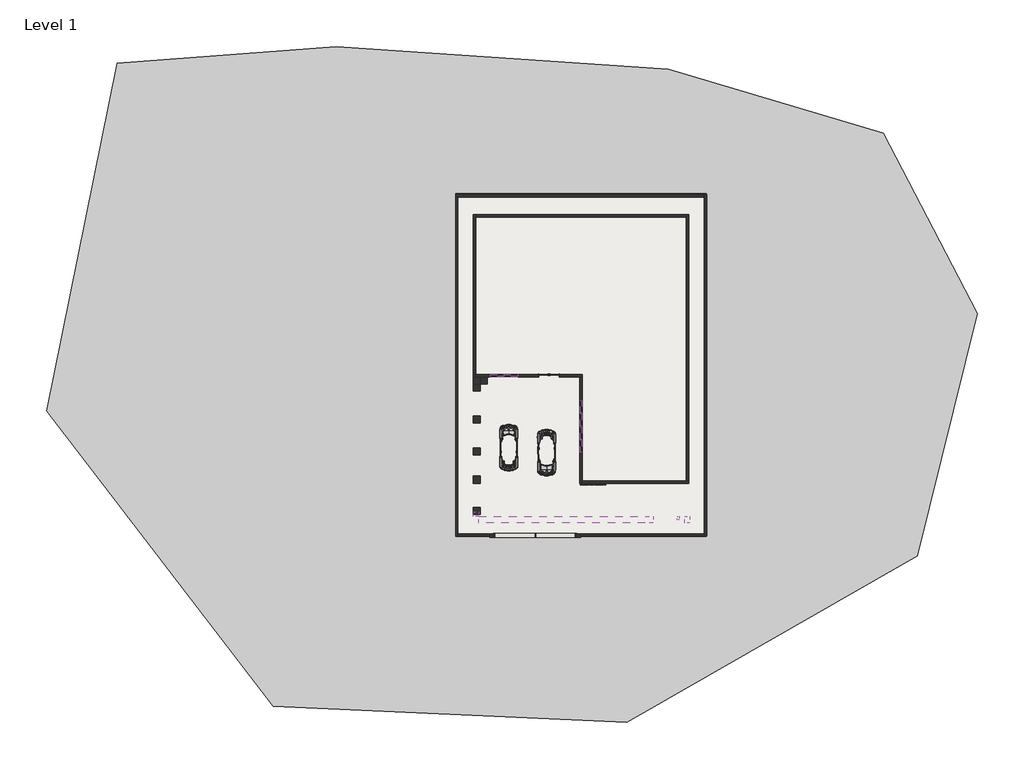
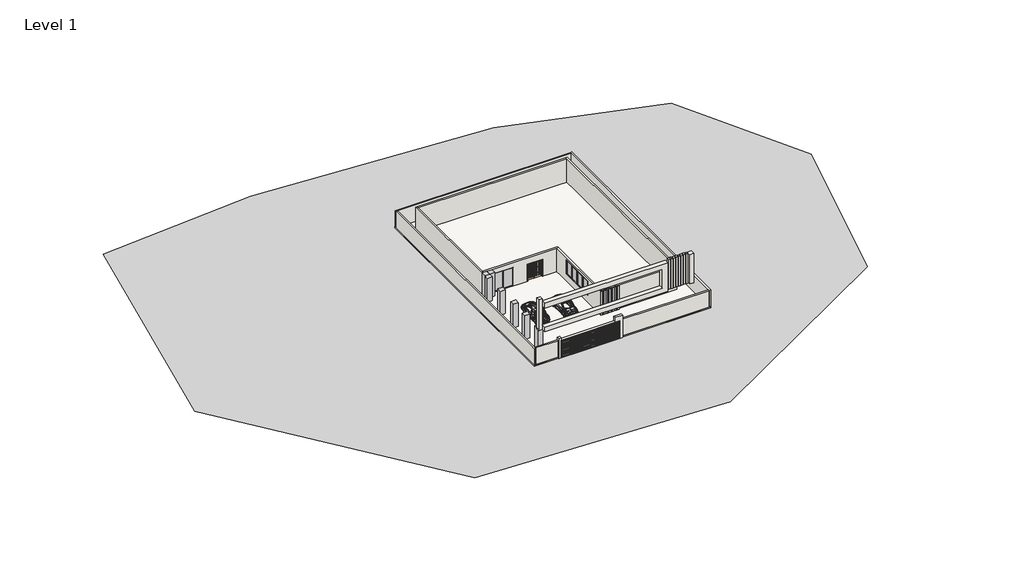
# One storey, incomplete: 20 members, 20 walls, 18 columns, 6 plates, 3 proxies, 1 door, 1 slab.
"""IFC4 building model written with IfcOpenShell, lengths in millimetres."""

from ifc_helpers import new_model, si_unit, frame, origin, origin_with_axes, place, context, project, spatial, polyline, outline, extrude, faceted_brep, triangles, transform, mapped, element, save
from components import rpc_beetle_rpc_beetle_3ce7ba48, m_rectangular_column_610_x_610mm_b887bf16, door_2f318157, rectangular_mullion_50_x_150mm_a98d9a75, rectangular_mullion_50_x_150mm_4a8db126, rectangular_mullion_50_x_150mm_7b2d4eb8, rectangular_mullion_50_x_150mm_561fbe3c, rectangular_mullion_50_x_150mm_8c42de37, rectangular_mullion_50_x_150mm_71d0ff5f, rectangular_mullion_50_x_150mm_c76b6149, system_panel_glazed_3787533d, system_panel_glazed_0469dc57, system_panel_glazed_71021e01, walls_1_walls_1_ac2cf788, walls_10_walls_9_f4ffd68b, walls_2_walls_2_f87d77c0, walls_4_walls_1_0671908a, walls_5_walls_5_96d48458, walls_6_walls_6_895ef20a, walls_7_walls_7_225e37e1, walls_8_walls_8_394d44dd, walls_9_walls_9_57911b2c

model = new_model("IFC4")

# Units and contexts
model_context = context("Model", 3, world=origin())
ifc_project = project(units=[si_unit("LENGTHUNIT", "METRE", prefix="MILLI")], contexts=[model_context])

# Site, building, storey
site = spatial("IfcSite", under=ifc_project)
building = spatial("IfcBuilding", under=site)
storey = spatial("IfcBuildingStorey", under=building, Name="Level 1", Elevation=0.0)

# Proxies
placement = place(None, origin())
element("IfcBuildingElementProxy", 1, Name="Building Element Proxy", at=placement, inside=storey, context=model_context, shape_type="Tessellation", body=[
    triangles([(-45355.9291992, -6804.9148682, -152.4), (-25904.1653503, -32148.7051208, -152.4), (4443.8121849, -33520.8213684, -152.4), (29384.0389893, -19234.671286, -152.4), (34549.651593, 1589.206921, -152.4), (26478.3814636, 17086.0466217, -152.4), (7995.171286, 22574.5104492, -152.4), (-20496.4140381, 24511.6154663, -152.4), (-39302.4754395, 23058.7878662, -152.4)], [[1, 2, 8], [8, 9, 1], [2, 3, 8], [3, 4, 7], [7, 5, 6], [5, 7, 4], [3, 7, 8]], closed=False),
])
rpc_beetle_rpc_beetle_shape = rpc_beetle_rpc_beetle_3ce7ba48(model_context)
element("IfcBuildingElementProxy", 2, Name="RPC Beetle : RPC Beetle", ObjectType="RPC Beetle : RPC Beetle", at=placement, inside=storey, context=model_context, shape_type="MappedRepresentation", body=[
    mapped(rpc_beetle_rpc_beetle_shape, transform((-5680.022521, -11169.2177849, 0.0), x_axis=(1.0, 0.0, 0.0), y_axis=(0.0, 1.0, 0.0), z_axis=(0.0, 0.0, 1.0))),
])
element("IfcBuildingElementProxy", 3, Name="RPC Beetle : RPC Beetle", ObjectType="RPC Beetle : RPC Beetle", at=placement, inside=storey, context=model_context, shape_type="MappedRepresentation", body=[
    mapped(rpc_beetle_rpc_beetle_shape, transform((-2432.022521, -9140.4177849, 0.0), x_axis=(-1.0000000000000004, 0.0, 0.0), y_axis=(0.0, -1.0000000000000004, 0.0), z_axis=(0.0, 0.0, 1.0))),
])

# Columns
element("IfcColumn", 4, ObjectType="M_Rectangular Column : 610 x 610mm", at=placement, inside=storey, context=model_context, shape_type="SweptSolid", body=[
    extrude(outline(polyline([(-8118.222521, -4463.8177849), (-8728.222521, -4463.8177849), (-8728.222521, -3853.8177849), (-8728.022521, -3853.8177849), (-8728.022521, -3854.0177849), (-8528.022521, -3854.0177849), (-8118.222521, -3854.0177849), (-8118.222521, -4463.8177849)])), origin_with_axes(), (0.0, 0.0, 1.0), 3048.0),
])
element("IfcColumn", 5, ObjectType="M_Rectangular Column : 610 x 610mm", at=placement, inside=storey, context=model_context, shape_type="SweptSolid", body=[
    extrude(outline(polyline([(-7508.622521, -4463.8177849), (-8118.622521, -4463.8177849), (-8118.622521, -3854.0177849), (-7508.622521, -3854.0177849), (-7508.622521, -4463.8177849)])), origin_with_axes(), (0.0, 0.0, 1.0), 3048.0),
])
m_rectangular_column_610_x_610mm_shape = m_rectangular_column_610_x_610mm_b887bf16(model_context)
element("IfcColumn", 6, ObjectType="M_Rectangular Column : 610 x 610mm", at=placement, inside=storey, context=model_context, shape_type="MappedRepresentation", body=[
    mapped(m_rectangular_column_610_x_610mm_shape, transform((-8423.222521, -4768.4177849, 0.0), x_axis=(1.0, 0.0, 0.0), y_axis=(0.0, 1.0, 0.0), z_axis=(0.0, 0.0, 1.0))),
])
element("IfcColumn", 7, ObjectType="M_Rectangular Column : 610 x 610mm", at=placement, inside=storey, context=model_context, shape_type="MappedRepresentation", body=[
    mapped(m_rectangular_column_610_x_610mm_shape, transform((-8423.222521, -7511.6177849, 0.0), x_axis=(1.0, 0.0, 0.0), y_axis=(0.0, 1.0, 0.0), z_axis=(0.0, 0.0, 1.0))),
])
element("IfcColumn", 8, ObjectType="M_Rectangular Column : 610 x 610mm", at=placement, inside=storey, context=model_context, shape_type="MappedRepresentation", body=[
    mapped(m_rectangular_column_610_x_610mm_shape, transform((-8423.222521, -10254.8177849, 0.0), x_axis=(1.0, 0.0, 0.0), y_axis=(0.0, 1.0, 0.0), z_axis=(0.0, 0.0, 1.0))),
])
element("IfcColumn", 9, ObjectType="M_Rectangular Column : 610 x 610mm", at=placement, inside=storey, context=model_context, shape_type="MappedRepresentation", body=[
    mapped(m_rectangular_column_610_x_610mm_shape, transform((-8423.222521, -12693.2177849, 0.0), x_axis=(1.0, 0.0, 0.0), y_axis=(0.0, 1.0, 0.0), z_axis=(0.0, 0.0, 1.0))),
])
element("IfcColumn", 10, ObjectType="M_Rectangular Column : 610 x 610mm", at=placement, inside=storey, context=model_context, shape_type="MappedRepresentation", body=[
    mapped(m_rectangular_column_610_x_610mm_shape, transform((-8423.222521, -15385.6177849, 0.0), x_axis=(1.0, 0.0, 0.0), y_axis=(0.0, 1.0, 0.0), z_axis=(0.0, 0.0, 1.0))),
])
element("IfcColumn", 11, ObjectType="M_Rectangular Column : COL 2", at=placement, inside=storey, context=model_context, shape_type="SweptSolid", body=[
    extrude(outline(polyline([(592.177479, -12998.0177849), (592.177479, -13150.4177849), (439.777479, -13150.4177849), (439.777479, -12998.0177849), (592.177479, -12998.0177849)])), origin_with_axes(), (0.0, 0.0, 1.0), 3048.0),
])
element("IfcColumn", 12, ObjectType="M_Rectangular Column : COL 2", at=placement, inside=storey, context=model_context, shape_type="SweptSolid", body=[
    extrude(outline(polyline([(793.777479, -12998.0177849), (793.777479, -13150.4177849), (641.377479, -13150.4177849), (641.377479, -12998.0177849), (793.777479, -12998.0177849)])), origin_with_axes(), (0.0, 0.0, 1.0), 3048.0),
])
element("IfcColumn", 13, ObjectType="M_Rectangular Column : COL 2", at=placement, inside=storey, context=model_context, shape_type="SweptSolid", body=[
    extrude(outline(polyline([(996.977479, -12998.0177849), (996.977479, -13150.4177849), (844.577479, -13150.4177849), (844.577479, -12998.0177849), (996.977479, -12998.0177849)])), origin_with_axes(), (0.0, 0.0, 1.0), 3048.0),
])
element("IfcColumn", 14, ObjectType="M_Rectangular Column : COL 2", at=placement, inside=storey, context=model_context, shape_type="SweptSolid", body=[
    extrude(outline(polyline([(1200.177479, -12998.0177849), (1200.177479, -13150.4177849), (1047.777479, -13150.4177849), (1047.777479, -12998.0177849), (1200.177479, -12998.0177849)])), origin_with_axes(), (0.0, 0.0, 1.0), 3048.0),
])
element("IfcColumn", 15, ObjectType="M_Rectangular Column : COL 2", at=placement, inside=storey, context=model_context, shape_type="SweptSolid", body=[
    extrude(outline(polyline([(1403.377479, -12998.0177849), (1403.377479, -13150.4177849), (1250.977479, -13150.4177849), (1250.977479, -12998.0177849), (1403.377479, -12998.0177849)])), origin_with_axes(), (0.0, 0.0, 1.0), 3048.0),
])
element("IfcColumn", 16, ObjectType="M_Rectangular Column : COL 2", at=placement, inside=storey, context=model_context, shape_type="SweptSolid", body=[
    extrude(outline(polyline([(1606.577479, -12998.0177849), (1606.577479, -13150.4177849), (1454.177479, -13150.4177849), (1454.177479, -12998.0177849), (1606.577479, -12998.0177849)])), origin_with_axes(), (0.0, 0.0, 1.0), 3048.0),
])
element("IfcColumn", 17, ObjectType="M_Rectangular Column : COL 2", at=placement, inside=storey, context=model_context, shape_type="SweptSolid", body=[
    extrude(outline(polyline([(1835.177479, -12998.0177849), (1835.177479, -13150.4177849), (1682.777479, -13150.4177849), (1682.777479, -12998.0177849), (1835.177479, -12998.0177849)])), origin_with_axes(), (0.0, 0.0, 1.0), 3048.0),
])
element("IfcColumn", 18, ObjectType="M_Rectangular Column : COL 2", at=placement, inside=storey, context=model_context, shape_type="SweptSolid", body=[
    extrude(outline(polyline([(2038.377479, -12998.0177849), (2038.377479, -13150.4177849), (1885.977479, -13150.4177849), (1885.977479, -12998.0177849), (2038.377479, -12998.0177849)])), origin_with_axes(), (0.0, 0.0, 1.0), 3048.0),
])
element("IfcColumn", 19, ObjectType="M_Rectangular Column : COL 2", at=placement, inside=storey, context=model_context, shape_type="SweptSolid", body=[
    extrude(outline(polyline([(2241.577479, -12998.0177849), (2241.577479, -13150.4177849), (2089.177479, -13150.4177849), (2089.177479, -12998.0177849), (2241.577479, -12998.0177849)])), origin_with_axes(), (0.0, 0.0, 1.0), 3048.0),
])
element("IfcColumn", 20, ObjectType="M_Rectangular Column : COL 2", at=placement, inside=storey, context=model_context, shape_type="SweptSolid", body=[
    extrude(outline(polyline([(2444.777479, -12998.0177849), (2444.777479, -13150.4177849), (2292.377479, -13150.4177849), (2292.377479, -12998.0177849), (2444.777479, -12998.0177849)])), origin_with_axes(), (0.0, 0.0, 1.0), 3048.0),
])
element("IfcColumn", 21, ObjectType="M_Rectangular Column : COL 2", at=placement, inside=storey, context=model_context, shape_type="SweptSolid", body=[
    extrude(outline(polyline([(2647.977479, -12998.0177849), (2647.977479, -13150.4177849), (2495.577479, -13150.4177849), (2495.577479, -12998.0177849), (2647.977479, -12998.0177849)])), origin_with_axes(), (0.0, 0.0, 1.0), 3048.0),
])

# Door
door_shape = door_2f318157(model_context)
element("IfcDoor", 22, ObjectType="Door-Interior-Double-Full Glass-Wood : 68\" x 84\"", at=placement, inside=storey, context=model_context, shape_type="MappedRepresentation", body=[
    mapped(door_shape, transform((-2227.222521, -3750.8427849, 0.0), x_axis=(1.0, 0.0, 0.0), y_axis=(0.0, 1.0, 0.0), z_axis=(0.0, 0.0, 1.0))),
])

# Members
rectangular_mullion_50_x_150mm_shape = rectangular_mullion_50_x_150mm_a98d9a75(model_context)
element("IfcMember", 23, ObjectType="Rectangular Mullion : 50 x 150mm", at=placement, inside=storey, context=model_context, shape_type="MappedRepresentation", body=[
    mapped(rectangular_mullion_50_x_150mm_shape, transform((-6089.622521, -3754.0177849, 0.0), x_axis=(1.0, 0.0, 0.0), y_axis=(0.0, -1.0, 0.0), z_axis=(0.0, 0.0, -1.0))),
])
rectangular_mullion_50_x_150mm_2_shape = rectangular_mullion_50_x_150mm_4a8db126(model_context)
element("IfcMember", 24, ObjectType="Rectangular Mullion : 50 x 150mm", at=placement, inside=storey, context=model_context, shape_type="MappedRepresentation", body=[
    mapped(rectangular_mullion_50_x_150mm_2_shape, transform((-7308.822521, -3754.0177849, 2438.4), x_axis=(-1.0, 0.0, 0.0), y_axis=(0.0, -1.0, 0.0), z_axis=(0.0, 0.0, 1.0))),
])
element("IfcMember", 25, ObjectType="Rectangular Mullion : 50 x 150mm", at=placement, inside=storey, context=model_context, shape_type="MappedRepresentation", body=[
    mapped(rectangular_mullion_50_x_150mm_2_shape, transform((-4870.422521, -3754.0177849, 0.0), x_axis=(1.0, 0.0, 0.0), y_axis=(0.0, -1.0, 0.0), z_axis=(0.0, 0.0, -1.0))),
])
rectangular_mullion_50_x_150mm_3_shape = rectangular_mullion_50_x_150mm_7b2d4eb8(model_context)
element("IfcMember", 26, ObjectType="Rectangular Mullion : 50 x 150mm", at=placement, inside=storey, context=model_context, shape_type="MappedRepresentation", body=[
    mapped(rectangular_mullion_50_x_150mm_3_shape, transform((-4920.422521, -3754.0177849, 2438.4), x_axis=(0.0, 0.0, 1.0), y_axis=(0.0, -1.0, 0.0), z_axis=(1.0, 0.0, 0.0))),
])
element("IfcMember", 27, ObjectType="Rectangular Mullion : 50 x 150mm", at=placement, inside=storey, context=model_context, shape_type="MappedRepresentation", body=[
    mapped(rectangular_mullion_50_x_150mm_3_shape, transform((-6114.622521, -3754.0177849, 2438.4), x_axis=(0.0, 0.0, 1.0), y_axis=(0.0, -1.0, 0.0), z_axis=(1.0, 0.0, 0.0))),
])
element("IfcMember", 28, ObjectType="Rectangular Mullion : 50 x 150mm", at=placement, inside=storey, context=model_context, shape_type="MappedRepresentation", body=[
    mapped(rectangular_mullion_50_x_150mm_3_shape, transform((-7258.822521, -3754.0177849, 0.0), x_axis=(0.0, 0.0, -1.0), y_axis=(0.0, -1.0, 0.0), z_axis=(-1.0, 0.0, 0.0))),
])
element("IfcMember", 29, ObjectType="Rectangular Mullion : 50 x 150mm", at=placement, inside=storey, context=model_context, shape_type="MappedRepresentation", body=[
    mapped(rectangular_mullion_50_x_150mm_3_shape, transform((-6064.622521, -3754.0177849, 0.0), x_axis=(0.0, 0.0, -1.0), y_axis=(0.0, -1.0, 0.0), z_axis=(-1.0, 0.0, 0.0))),
])
rectangular_mullion_50_x_150mm_4_shape = rectangular_mullion_50_x_150mm_561fbe3c(model_context)
element("IfcMember", 30, ObjectType="Rectangular Mullion : 50 x 150mm", at=placement, inside=storey, context=model_context, shape_type="MappedRepresentation", body=[
    mapped(rectangular_mullion_50_x_150mm_4_shape, transform((515.977479, -10357.2177849, 2743.2), x_axis=(0.0, 0.0, 1.0), y_axis=(-1.0, 0.0, 0.0), z_axis=(0.0, -1.0, 0.0))),
])
element("IfcMember", 31, ObjectType="Rectangular Mullion : 50 x 150mm", at=placement, inside=storey, context=model_context, shape_type="MappedRepresentation", body=[
    mapped(rectangular_mullion_50_x_150mm_4_shape, transform((515.977479, -6953.2177849, 2743.2), x_axis=(0.0, 0.0, 1.0), y_axis=(-1.0, 0.0, 0.0), z_axis=(0.0, -1.0, 0.0))),
])
element("IfcMember", 32, ObjectType="Rectangular Mullion : 50 x 150mm", at=placement, inside=storey, context=model_context, shape_type="MappedRepresentation", body=[
    mapped(rectangular_mullion_50_x_150mm_4_shape, transform((515.977479, -5885.2177849, 914.4), x_axis=(0.0, 0.0, -1.0), y_axis=(-1.0, 0.0, 0.0), z_axis=(0.0, 1.0, 0.0))),
])
element("IfcMember", 33, ObjectType="Rectangular Mullion : 50 x 150mm", at=placement, inside=storey, context=model_context, shape_type="MappedRepresentation", body=[
    mapped(rectangular_mullion_50_x_150mm_4_shape, transform((515.977479, -9289.2177849, 914.4), x_axis=(0.0, 0.0, -1.0), y_axis=(-1.0, 0.0, 0.0), z_axis=(0.0, 1.0, 0.0))),
])
rectangular_mullion_50_x_150mm_5_shape = rectangular_mullion_50_x_150mm_8c42de37(model_context)
element("IfcMember", 34, ObjectType="Rectangular Mullion : 50 x 150mm", at=placement, inside=storey, context=model_context, shape_type="MappedRepresentation", body=[
    mapped(rectangular_mullion_50_x_150mm_5_shape, transform((515.977479, -8121.2177849, 914.4), x_axis=(0.0, -1.0, 0.0), y_axis=(-1.0, 0.0, 0.0), z_axis=(0.0, 0.0, -1.0))),
])
element("IfcMember", 35, ObjectType="Rectangular Mullion : 50 x 150mm", at=placement, inside=storey, context=model_context, shape_type="MappedRepresentation", body=[
    mapped(rectangular_mullion_50_x_150mm_5_shape, transform((515.977479, -6978.2177849, 914.4), x_axis=(0.0, -1.0, 0.0), y_axis=(-1.0, 0.0, 0.0), z_axis=(0.0, 0.0, -1.0))),
])
element("IfcMember", 36, ObjectType="Rectangular Mullion : 50 x 150mm", at=placement, inside=storey, context=model_context, shape_type="MappedRepresentation", body=[
    mapped(rectangular_mullion_50_x_150mm_5_shape, transform((515.977479, -9264.2177849, 914.4), x_axis=(0.0, -1.0, 0.0), y_axis=(-1.0, 0.0, 0.0), z_axis=(0.0, 0.0, -1.0))),
])
rectangular_mullion_50_x_150mm_6_shape = rectangular_mullion_50_x_150mm_71d0ff5f(model_context)
element("IfcMember", 37, ObjectType="Rectangular Mullion : 50 x 150mm", at=placement, inside=storey, context=model_context, shape_type="MappedRepresentation", body=[
    mapped(rectangular_mullion_50_x_150mm_6_shape, transform((515.977479, -8146.2177849, 914.4), x_axis=(0.0, 0.0, -1.0), y_axis=(-1.0, 0.0, 0.0), z_axis=(0.0, 1.0, 0.0))),
])
element("IfcMember", 38, ObjectType="Rectangular Mullion : 50 x 150mm", at=placement, inside=storey, context=model_context, shape_type="MappedRepresentation", body=[
    mapped(rectangular_mullion_50_x_150mm_6_shape, transform((515.977479, -7003.2177849, 914.4), x_axis=(0.0, 0.0, -1.0), y_axis=(-1.0, 0.0, 0.0), z_axis=(0.0, 1.0, 0.0))),
])
element("IfcMember", 39, ObjectType="Rectangular Mullion : 50 x 150mm", at=placement, inside=storey, context=model_context, shape_type="MappedRepresentation", body=[
    mapped(rectangular_mullion_50_x_150mm_6_shape, transform((515.977479, -8096.2177849, 2743.2), x_axis=(0.0, 0.0, 1.0), y_axis=(-1.0, 0.0, 0.0), z_axis=(0.0, -1.0, 0.0))),
])
element("IfcMember", 40, ObjectType="Rectangular Mullion : 50 x 150mm", at=placement, inside=storey, context=model_context, shape_type="MappedRepresentation", body=[
    mapped(rectangular_mullion_50_x_150mm_6_shape, transform((515.977479, -9239.2177849, 2743.2), x_axis=(0.0, 0.0, 1.0), y_axis=(-1.0, 0.0, 0.0), z_axis=(0.0, -1.0, 0.0))),
])
rectangular_mullion_50_x_150mm_7_shape = rectangular_mullion_50_x_150mm_c76b6149(model_context)
element("IfcMember", 41, ObjectType="Rectangular Mullion : 50 x 150mm", at=placement, inside=storey, context=model_context, shape_type="MappedRepresentation", body=[
    mapped(rectangular_mullion_50_x_150mm_7_shape, transform((515.977479, -5835.2177849, 2743.2), x_axis=(0.0, 1.0, 0.0), y_axis=(-1.0, 0.0, 0.0), z_axis=(0.0, 0.0, 1.0))),
])
element("IfcMember", 42, ObjectType="Rectangular Mullion : 50 x 150mm", at=placement, inside=storey, context=model_context, shape_type="MappedRepresentation", body=[
    mapped(rectangular_mullion_50_x_150mm_7_shape, transform((515.977479, -10407.2177849, 914.4), x_axis=(0.0, -1.0, 0.0), y_axis=(-1.0, 0.0, 0.0), z_axis=(0.0, 0.0, -1.0))),
])

# Plates
system_panel_glazed_shape = system_panel_glazed_3787533d(model_context)
element("IfcPlate", 43, ObjectType="System Panel : Glazed", at=placement, inside=storey, context=model_context, shape_type="MappedRepresentation", body=[
    mapped(system_panel_glazed_shape, transform((-6686.722521, -3754.0177849, 50.0), x_axis=(1.0, 0.0, 0.0), y_axis=(0.0, 1.0, 0.0), z_axis=(0.0, 0.0, 1.0))),
])
element("IfcPlate", 44, ObjectType="System Panel : Glazed", at=placement, inside=storey, context=model_context, shape_type="MappedRepresentation", body=[
    mapped(system_panel_glazed_shape, transform((-5492.522521, -3754.0177849, 50.0), x_axis=(1.0, 0.0, 0.0), y_axis=(0.0, 1.0, 0.0), z_axis=(0.0, 0.0, 1.0))),
])
system_panel_glazed_2_shape = system_panel_glazed_0469dc57(model_context)
element("IfcPlate", 45, ObjectType="System Panel : Glazed", at=placement, inside=storey, context=model_context, shape_type="MappedRepresentation", body=[
    mapped(system_panel_glazed_2_shape, transform((515.977479, -6419.2177849, 964.4), x_axis=(0.0, -1.0, 0.0), y_axis=(1.0, 0.0, 0.0), z_axis=(0.0, 0.0, 1.0))),
])
element("IfcPlate", 46, ObjectType="System Panel : Glazed", at=placement, inside=storey, context=model_context, shape_type="MappedRepresentation", body=[
    mapped(system_panel_glazed_2_shape, transform((515.977479, -9823.2177849, 964.4), x_axis=(0.0, -1.0, 0.0), y_axis=(1.0, 0.0, 0.0), z_axis=(0.0, 0.0, 1.0))),
])
system_panel_glazed_3_shape = system_panel_glazed_71021e01(model_context)
element("IfcPlate", 47, ObjectType="System Panel : Glazed", at=placement, inside=storey, context=model_context, shape_type="MappedRepresentation", body=[
    mapped(system_panel_glazed_3_shape, transform((515.977479, -8692.7177849, 964.4), x_axis=(0.0, -1.0, 0.0), y_axis=(1.0, 0.0, 0.0), z_axis=(0.0, 0.0, 1.0))),
])
element("IfcPlate", 48, ObjectType="System Panel : Glazed", at=placement, inside=storey, context=model_context, shape_type="MappedRepresentation", body=[
    mapped(system_panel_glazed_3_shape, transform((515.977479, -7549.7177849, 964.4), x_axis=(0.0, -1.0, 0.0), y_axis=(1.0, 0.0, 0.0), z_axis=(0.0, 0.0, 1.0))),
])

# Slab
element("IfcSlab", 49, ObjectType="Generic 150mm", at=placement, inside=storey, context=model_context, shape_type="SweptSolid", body=[
    extrude(outline(polyline([(-10252.022521, 11890.7822151), (11283.977479, 11890.7822151), (11283.977479, -17570.0177849), (-10252.022521, -17570.0177849), (-10252.022521, 11890.7822151)])), frame((0.0, 0.0, -152.4), z_axis=(0.0, 0.0, 1.0), x_axis=(1.0, 0.0, 0.0)), (0.0, 0.0, 1.0), 152.4),
])

# Walls
element("IfcWall", 50, ObjectType="Generic - 200mm", at=placement, inside=storey, context=model_context, shape_type="Brep", body=[
    faceted_brep([(-8728.022521, 10061.9822151, 0.0), (-8728.022521, -3853.8177849, 0.0), (-8728.022521, -3854.0177849, 0.0), (-8728.022521, -3854.0177849, 3048.0), (-8728.022521, -3853.8177849, 3048.0), (-8728.022521, 10061.9822151, 3048.0), (-8528.022521, 10061.9822151, 0.0), (-8528.022521, 10061.9822151, 3048.0), (-8528.022521, 9861.9822151, 3048.0), (-8528.022521, -3654.0177849, 3048.0), (-8528.022521, -3854.0177849, 3048.0), (-8528.022521, -3854.0177849, 0.0), (-8528.022521, -3654.0177849, 0.0), (-8528.022521, 9861.9822151, 0.0)], [[[0, 1, 2, 3, 4, 5]], [[6, 7, 8, 9, 10, 11, 12, 13]], [[2, 1, 0, 6, 13, 12, 11]], [[5, 4, 3, 10, 9, 8, 7]], [[3, 2, 11, 10]], [[0, 5, 7, 6]]]),
])
element("IfcWall", 51, ObjectType="Generic - 200mm", at=placement, inside=storey, context=model_context, shape_type="Brep", body=[
    faceted_brep([(615.977479, -3854.0177849, 3048.0), (415.977479, -3854.0177849, 3048.0), (-7508.622521, -3854.0177849, 3048.0), (-8118.222521, -3854.0177849, 3048.0), (-8118.622521, -3854.0177849, 3048.0), (-8528.022521, -3854.0177849, 3048.0), (-8528.022521, -3854.0177849, 0.0), (-8118.622521, -3854.0177849, 0.0), (-8118.222521, -3854.0177849, 0.0), (-7508.622521, -3854.0177849, 0.0), (-7308.822521, -3854.0177849, 0.0), (-7308.822521, -3854.0177849, 2438.4), (-4870.422521, -3854.0177849, 2438.4), (-4870.422521, -3854.0177849, 0.0), (-3116.222521, -3854.0177849, 0.0), (-3116.222521, -3854.0177849, 2159.0), (-1338.222521, -3854.0177849, 2159.0), (-1338.222521, -3854.0177849, 0.0), (415.977479, -3854.0177849, 0.0), (615.977479, -3854.0177849, 0.0), (-8528.022521, -3654.0177849, 3048.0), (615.977479, -3654.0177849, 3048.0), (615.977479, -3654.0177849, 0.0), (-1338.222521, -3654.0177849, 0.0), (-1338.222521, -3654.0177849, 2159.0), (-3116.222521, -3654.0177849, 2159.0), (-3116.222521, -3654.0177849, 0.0), (-4870.422521, -3654.0177849, 0.0), (-4870.422521, -3654.0177849, 2438.4), (-7308.822521, -3654.0177849, 2438.4), (-7308.822521, -3654.0177849, 0.0), (-8528.022521, -3654.0177849, 0.0)], [[[0, 1, 2, 3, 4, 5, 6, 7, 8, 9, 10, 11, 12, 13, 14, 15, 16, 17, 18, 19]], [[20, 21, 22, 23, 24, 25, 26, 27, 28, 29, 30, 31]], [[6, 31, 30, 10, 9, 8, 7]], [[22, 19, 18, 17, 23]], [[13, 27, 26, 14]], [[5, 4, 3, 2, 1, 0, 21, 20]], [[6, 5, 20, 31]], [[0, 19, 22, 21]], [[29, 11, 10, 30]], [[11, 29, 28, 12]], [[12, 28, 27, 13]], [[16, 24, 23, 17]], [[24, 16, 15, 25]], [[25, 15, 14, 26]]]),
])
element("IfcWall", 52, ObjectType="Generic - 200mm", at=placement, inside=storey, context=model_context, shape_type="Brep", body=[
    faceted_brep([(415.977479, -3854.0177849, 0.0), (415.977479, -12998.0177849, 0.0), (415.977479, -12998.0177849, 3048.0), (415.977479, -3854.0177849, 3048.0), (415.977479, -5835.2177849, 914.4), (415.977479, -5835.2177849, 2743.2), (415.977479, -10407.2177849, 2743.2), (415.977479, -10407.2177849, 914.4), (615.977479, -12998.0177849, 0.0), (615.977479, -12798.0177849, 0.0), (615.977479, -3854.0177849, 0.0), (615.977479, -3854.0177849, 3048.0), (615.977479, -12798.0177849, 3048.0), (615.977479, -12998.0177849, 3048.0), (615.977479, -5835.2177849, 2743.2), (615.977479, -5835.2177849, 914.4), (615.977479, -10407.2177849, 914.4), (615.977479, -10407.2177849, 2743.2), (592.177479, -12998.0177849, 0.0), (439.777479, -12998.0177849, 0.0), (439.777479, -12998.0177849, 3048.0), (592.177479, -12998.0177849, 3048.0)], [[[0, 1, 2, 3], [4, 5, 6, 7]], [[8, 9, 10, 11, 12, 13], [14, 15, 16, 17]], [[1, 0, 10, 9, 8, 18, 19]], [[3, 2, 20, 21, 13, 12, 11]], [[0, 3, 11, 10]], [[2, 1, 19, 18, 8, 13, 21, 20]], [[4, 15, 14, 5]], [[5, 14, 17, 6]], [[6, 17, 16, 7]], [[15, 4, 7, 16]]]),
])
element("IfcWall", 53, ObjectType="Generic - 200mm", at=placement, inside=storey, context=model_context, shape_type="Brep", body=[
    faceted_brep([(615.977479, -12998.0177849, 0.0), (641.377479, -12998.0177849, 0.0), (793.777479, -12998.0177849, 0.0), (844.577479, -12998.0177849, 0.0), (996.977479, -12998.0177849, 0.0), (1047.777479, -12998.0177849, 0.0), (1200.177479, -12998.0177849, 0.0), (1250.977479, -12998.0177849, 0.0), (1403.377479, -12998.0177849, 0.0), (1454.177479, -12998.0177849, 0.0), (1606.577479, -12998.0177849, 0.0), (1682.777479, -12998.0177849, 0.0), (1835.177479, -12998.0177849, 0.0), (1885.977479, -12998.0177849, 0.0), (2038.377479, -12998.0177849, 0.0), (2089.177479, -12998.0177849, 0.0), (2241.577479, -12998.0177849, 0.0), (2292.377479, -12998.0177849, 0.0), (2444.777479, -12998.0177849, 0.0), (2495.577479, -12998.0177849, 0.0), (2647.977479, -12998.0177849, 0.0), (9759.977479, -12998.0177849, 0.0), (9759.977479, -12998.0177849, 3048.0), (2647.977479, -12998.0177849, 3048.0), (2495.577479, -12998.0177849, 3048.0), (2444.777479, -12998.0177849, 3048.0), (2292.377479, -12998.0177849, 3048.0), (2241.577479, -12998.0177849, 3048.0), (2089.177479, -12998.0177849, 3048.0), (2038.377479, -12998.0177849, 3048.0), (1885.977479, -12998.0177849, 3048.0), (1835.177479, -12998.0177849, 3048.0), (1682.777479, -12998.0177849, 3048.0), (1606.577479, -12998.0177849, 3048.0), (1454.177479, -12998.0177849, 3048.0), (1403.377479, -12998.0177849, 3048.0), (1250.977479, -12998.0177849, 3048.0), (1200.177479, -12998.0177849, 3048.0), (1047.777479, -12998.0177849, 3048.0), (996.977479, -12998.0177849, 3048.0), (844.577479, -12998.0177849, 3048.0), (793.777479, -12998.0177849, 3048.0), (641.377479, -12998.0177849, 3048.0), (615.977479, -12998.0177849, 3048.0), (615.977479, -12798.0177849, 0.0), (615.977479, -12798.0177849, 3048.0), (9559.977479, -12798.0177849, 3048.0), (9759.977479, -12798.0177849, 3048.0), (9759.977479, -12798.0177849, 0.0), (9559.977479, -12798.0177849, 0.0)], [[[0, 1, 2, 3, 4, 5, 6, 7, 8, 9, 10, 11, 12, 13, 14, 15, 16, 17, 18, 19, 20, 21, 22, 23, 24, 25, 26, 27, 28, 29, 30, 31, 32, 33, 34, 35, 36, 37, 38, 39, 40, 41, 42, 43]], [[44, 45, 46, 47, 48, 49]], [[21, 20, 19, 18, 17, 16, 15, 14, 13, 12, 11, 10, 9, 8, 7, 6, 5, 4, 3, 2, 1, 0, 44, 49, 48]], [[43, 42, 41, 40, 39, 38, 37, 36, 35, 34, 33, 32, 31, 30, 29, 28, 27, 26, 25, 24, 23, 22, 47, 46, 45]], [[0, 43, 45, 44]], [[22, 21, 48, 47]]]),
])
element("IfcWall", 54, ObjectType="Generic - 200mm", at=placement, inside=storey, context=model_context, shape_type="Brep", body=[
    faceted_brep([(9759.977479, -12798.0177849, 0.0), (9759.977479, 10061.9822151, 0.0), (9759.977479, 10061.9822151, 3048.0), (9759.977479, -12798.0177849, 3048.0), (9559.977479, -12798.0177849, 0.0), (9559.977479, -12798.0177849, 3048.0), (9559.977479, 9861.9822151, 3048.0), (9559.977479, 10061.9822151, 3048.0), (9559.977479, 10061.9822151, 0.0), (9559.977479, 9861.9822151, 0.0)], [[[0, 1, 2, 3]], [[4, 5, 6, 7, 8, 9]], [[1, 0, 4, 9, 8]], [[3, 2, 7, 6, 5]], [[0, 3, 5, 4]], [[2, 1, 8, 7]]]),
])
element("IfcWall", 55, ObjectType="Generic - 200mm", at=placement, inside=storey, context=model_context, shape_type="SweptSolid", body=[
    extrude(outline(polyline([(-8528.022521, 10061.9822151), (9559.977479, 10061.9822151), (9559.977479, 9861.9822151), (-8528.022521, 9861.9822151), (-8528.022521, 10061.9822151)])), origin_with_axes(), (0.0, 0.0, 1.0), 3048.0),
])
element("IfcWall", 56, ObjectType="Generic - 200mm", at=placement, inside=storey, context=model_context, shape_type="Brep", body=[
    faceted_brep([(11292.9366262, -17534.2834973, 0.0), (11292.9366262, 11774.1165027, 0.0), (11292.9366262, 11774.1165027, 2133.6), (11292.9366262, -17534.2834973, 2133.6), (11092.9366262, -17534.2834973, 0.0), (11092.9366262, -17534.2834973, 2133.6), (11092.9366262, -17334.2834973, 2133.6), (11092.9366262, 11574.1165027, 2133.6), (11092.9366262, 11774.1165027, 2133.6), (11092.9366262, 11774.1165027, 0.0), (11092.9366262, 11574.1165027, 0.0), (11092.9366262, -17334.2834973, 0.0)], [[[0, 1, 2, 3]], [[4, 5, 6, 7, 8, 9, 10, 11]], [[1, 0, 4, 11, 10, 9]], [[3, 2, 8, 7, 6, 5]], [[2, 1, 9, 8]], [[0, 3, 5, 4]]]),
])
element("IfcWall", 57, ObjectType="Generic - 200mm", at=placement, inside=storey, context=model_context, shape_type="Brep", body=[
    faceted_brep([(11092.9366262, 11774.1165027, 0.0), (-10243.0633738, 11774.1165027, 0.0), (-10243.0633738, 11774.1165027, 2133.6), (11092.9366262, 11774.1165027, 2133.6), (11092.9366262, 11574.1165027, 0.0), (11092.9366262, 11574.1165027, 2133.6), (-10043.0633738, 11574.1165027, 2133.6), (-10243.0633738, 11574.1165027, 2133.6), (-10243.0633738, 11574.1165027, 0.0), (-10043.0633738, 11574.1165027, 0.0)], [[[0, 1, 2, 3]], [[4, 5, 6, 7, 8, 9]], [[1, 0, 4, 9, 8]], [[3, 2, 7, 6, 5]], [[0, 3, 5, 4]], [[2, 1, 8, 7]]]),
])
element("IfcWall", 58, ObjectType="Generic - 200mm", at=placement, inside=storey, context=model_context, shape_type="Brep", body=[
    faceted_brep([(-10243.0633738, 11574.1165027, 0.0), (-10243.0633738, -17534.2834973, 0.0), (-10243.0633738, -17534.2834973, 2133.6), (-10243.0633738, 11574.1165027, 2133.6), (-10043.0633738, 11574.1165027, 0.0), (-10043.0633738, 11574.1165027, 2133.6), (-10043.0633738, -17334.2834973, 2133.6), (-10043.0633738, -17534.2834973, 2133.6), (-10043.0633738, -17534.2834973, 0.0), (-10043.0633738, -17334.2834973, 0.0)], [[[0, 1, 2, 3]], [[4, 5, 6, 7, 8, 9]], [[1, 0, 4, 9, 8]], [[3, 2, 7, 6, 5]], [[0, 3, 5, 4]], [[2, 1, 8, 7]]]),
])
element("IfcWall", 59, ObjectType="Generic - 200mm", at=placement, inside=storey, context=model_context, shape_type="SweptSolid", body=[
    extrude(outline(polyline([(-7308.822521, -17534.2834973), (-10043.0633738, -17534.2834973), (-10043.0633738, -17334.2834973), (-7308.822521, -17334.2834973), (-7308.822521, -17534.2834973)])), origin_with_axes(), (0.0, 0.0, 1.0), 2133.6),
])
element("IfcWall", 60, ObjectType="Generic - 200mm", at=placement, inside=storey, context=model_context, shape_type="SweptSolid", body=[
    extrude(outline(polyline([(515.977479, -17334.2834973), (11092.9366262, -17334.2834973), (11092.9366262, -17534.2834973), (515.977479, -17534.2834973), (515.977479, -17334.2834973)])), origin_with_axes(), (0.0, 0.0, 1.0), 2133.6),
])
walls_1_walls_1_shape = walls_1_walls_1_ac2cf788(model_context)
element("IfcWall", 61, ObjectType="Walls 1 : Walls 1", at=placement, inside=storey, context=model_context, shape_type="MappedRepresentation", body=[
    mapped(walls_1_walls_1_shape, transform((0.0, 0.0, 0.0), x_axis=(1.0, 0.0, 0.0), y_axis=(0.0, 1.0, 0.0), z_axis=(0.0, 0.0, 1.0))),
])
walls_10_walls_9_shape = walls_10_walls_9_f4ffd68b(model_context)
element("IfcWall", 62, ObjectType="Walls 10 : Walls 9", at=placement, inside=storey, context=model_context, shape_type="MappedRepresentation", body=[
    mapped(walls_10_walls_9_shape, transform((0.0, 0.0, 0.0), x_axis=(1.0, 0.0, 0.0), y_axis=(0.0, 1.0, 0.0), z_axis=(0.0, 0.0, 1.0))),
])
walls_2_walls_2_shape = walls_2_walls_2_f87d77c0(model_context)
element("IfcWall", 63, ObjectType="Walls 2 : Walls 2", at=placement, inside=storey, context=model_context, shape_type="MappedRepresentation", body=[
    mapped(walls_2_walls_2_shape, transform((0.0, 0.0, 0.0), x_axis=(1.0, 0.0, 0.0), y_axis=(0.0, 1.0, 0.0), z_axis=(0.0, 0.0, 1.0))),
])
walls_4_walls_1_shape = walls_4_walls_1_0671908a(model_context)
element("IfcWall", 64, ObjectType="Walls 4 : Walls 1", at=placement, inside=storey, context=model_context, shape_type="MappedRepresentation", body=[
    mapped(walls_4_walls_1_shape, transform((0.0, 0.0, 0.0), x_axis=(1.0, 0.0, 0.0), y_axis=(0.0, 1.0, 0.0), z_axis=(0.0, 0.0, 1.0))),
])
walls_5_walls_5_shape = walls_5_walls_5_96d48458(model_context)
element("IfcWall", 65, ObjectType="Walls 5 : Walls 5", at=placement, inside=storey, context=model_context, shape_type="MappedRepresentation", body=[
    mapped(walls_5_walls_5_shape, transform((0.0, 0.0, 0.0), x_axis=(1.0, 0.0, 0.0), y_axis=(0.0, 1.0, 0.0), z_axis=(0.0, 0.0, 1.0))),
])
walls_6_walls_6_shape = walls_6_walls_6_895ef20a(model_context)
element("IfcWall", 66, ObjectType="Walls 6 : Walls 6", at=placement, inside=storey, context=model_context, shape_type="MappedRepresentation", body=[
    mapped(walls_6_walls_6_shape, transform((0.0, 0.0, 0.0), x_axis=(1.0, 0.0, 0.0), y_axis=(0.0, 1.0, 0.0), z_axis=(0.0, 0.0, 1.0))),
])
walls_7_walls_7_shape = walls_7_walls_7_225e37e1(model_context)
element("IfcWall", 67, ObjectType="Walls 7 : Walls 7", at=placement, inside=storey, context=model_context, shape_type="MappedRepresentation", body=[
    mapped(walls_7_walls_7_shape, transform((0.0, 0.0, 0.0), x_axis=(1.0, 0.0, 0.0), y_axis=(0.0, 1.0, 0.0), z_axis=(0.0, 0.0, 1.0))),
])
walls_8_walls_8_shape = walls_8_walls_8_394d44dd(model_context)
element("IfcWall", 68, ObjectType="Walls 8 : Walls 8", at=placement, inside=storey, context=model_context, shape_type="MappedRepresentation", body=[
    mapped(walls_8_walls_8_shape, transform((0.0, 0.0, 0.0), x_axis=(1.0, 0.0, 0.0), y_axis=(0.0, 1.0, 0.0), z_axis=(0.0, 0.0, 1.0))),
])
walls_9_walls_9_shape = walls_9_walls_9_57911b2c(model_context)
element("IfcWall", 69, ObjectType="Walls 9 : Walls 9", at=placement, inside=storey, context=model_context, shape_type="MappedRepresentation", body=[
    mapped(walls_9_walls_9_shape, transform((0.0, 0.0, 0.0), x_axis=(1.0, 0.0, 0.0), y_axis=(0.0, 1.0, 0.0), z_axis=(0.0, 0.0, 1.0))),
])

save(model, "model.ifc")

# Revit data of these elements
# Type "RPC Beetle : RPC Beetle"
#   built-in parameter 1005195 = "RPC-16-0U6E-L4EG-ENH1-J3KF-SVEL-0TX4-C0"
#   Height = 0
# Type "M_Rectangular Column : 610 x 610mm"
#   Depth = 610 mm
#   Offset Base = 0 mm
#   Offset Top = 0 mm
#   Width = 610 mm
#   Material = none
# Type "M_Rectangular Column : COL 2"
#   Depth = 152.4 mm
#   Offset Base = 0 mm
#   Offset Top = 0 mm
#   Width = 152.4 mm
#   Material = none
# Type "Door-Interior-Double-Full Glass-Wood : 68\" x 84\""
#   Type Mark = "40"
#   Assembly Code = "C1020300"
#   Analytic Construction = "French door, wood frame with single glass"
#   Top Rail = 119.063 mm
#   Thickness = 34.925 mm
#   Thermal Resistance (R) = 0.188367 (m²·K)/W
#   Swing Angle [instance default] = 90.00°
#   Stiles = 120.65 mm
#   Rough Width = 1778 mm
#   Rough Height = 2159 mm
#   Panel Width = 863.6 mm
#   Height = 2133.6 mm
#   Width = 1727.2 mm
#   Heat Transfer Coefficient (U) = 5.30918 W/(m²·K)
#   Bottom Rail = 231.775 mm
#   Show Grill [instance default] = yes
#   Trim Material = Cherry
#   Panel Material = Cherry
#   Frame Material = Cherry
#   Door Handle Material = Aluminum
#   Visual Light Transmittance = 0
#   Solar Heat Gain Coefficient = 0
#   Wall Closure = (empty or 0)
#   Function = (empty or 0)
# Type "Rectangular Mullion : 50 x 150mm"
#   built-in parameter 1007304 = 0.492126 (stored number, unit not read)
#   built-in parameter 1007301 = 0.082021 (stored number, unit not read)
#   built-in parameter 1007300 = 0.082021 (stored number, unit not read)
# Type "System Panel : Glazed"
#   Construction Type Id = "GSP4R"
#   Analytic Construction = "1/8 in Pilkington single glazing"
#   Visual Light Transmittance = 0.9
#   Solar Heat Gain Coefficient = 0.86
#   Heat Transfer Coefficient (U) = 6.7069 W/(m²·K)
# Type "Generic 150mm"
#   Function = 0
#   Layers, outside or top first: 152.4 mm no material (function 1)
# Type "Generic - 200mm"
#   Layers, outside or top first: 200 mm no material (function 1)
# Element 1 (IfcBuildingElementProxy)
#   Material = none
#   Phase Created = New Construction
# Elements 2, 3 (IfcBuildingElementProxy, "RPC Beetle : RPC Beetle")
#   Phase Created = New Construction
# Element 4 (IfcColumn, "M_Rectangular Column : 610 x 610mm")
#   Phase Created = New Construction
#   Materials on its faces: "Default Wall", "CREAM WALL", "Door - Handle"
# Element 5 (IfcColumn, "M_Rectangular Column : 610 x 610mm")
#   Phase Created = New Construction
#   Materials on its faces: "CREAM WALL", "Default Wall"
# Elements 6, 7, 8, 9, 10 (IfcColumn, "M_Rectangular Column : 610 x 610mm")
#   Phase Created = New Construction
# Element 11 (IfcColumn, "M_Rectangular Column : COL 2")
#   Phase Created = New Construction
#   Materials on its faces: "Sash", "Default Wall", "Oak Flooring"
# Elements 12, 13, 14, 15, 16, 17, 18, 19, 20, 21 (IfcColumn, "M_Rectangular Column : COL 2")
#   Phase Created = New Construction
#   Materials on its faces: "Sash", "Default Wall"
# Element 22 (IfcDoor, "Door-Interior-Double-Full Glass-Wood : 68\" x 84\"")
#   Swing Angle = 90.00°
#   Show Grill = yes
#   Phase Created = New Construction
#   Materials on its faces: "Cherry", "Aluminum", "Glass"
# Elements 23, 24, 25, 26, 27, 28, 29, 30, 31, 32, 33, 34, 35, 36, 37, 38, 39, 40, 41, 42 (IfcMember, "Rectangular Mullion : 50 x 150mm")
#   Phase Created = New Construction
#   Materials on its faces: "Aluminium"
# Elements 43, 44, 45, 46, 47, 48 (IfcPlate, "System Panel : Glazed")
#   Phase Created = New Construction
#   Materials on its faces: "Glass"
# Element 49 (IfcSlab, "Generic 150mm")
#   built-in parameter 1001955 = 3.14159 (stored number, unit not read)
#   Height Offset From Level = 0 mm
#   Phase Created = New Construction
#   Materials on its faces: "Default Floor", "Ceiling Tile 600 x 600", "Door - Frame"
# Elements 50, 51, 53, 54 (IfcWall, "Generic - 200mm")
#   Top Offset = 0 mm
#   Base Offset = 0 mm
#   Unconnected Height = 3048 mm
#   wall height = 3048 mm
#   Phase Created = New Construction
#   Base Constraint = Level 1
#   Materials on its faces: "Default Wall", "CREAM WALL"
# Element 52 (IfcWall, "Generic - 200mm")
#   Top Offset = 0 mm
#   Base Offset = 0 mm
#   Unconnected Height = 3048 mm
#   wall height = 3048 mm
#   Phase Created = New Construction
#   Base Constraint = Level 1
#   Materials on its faces: "Default Wall", "CREAM WALL", "Oak Flooring"
# Element 55 (IfcWall, "Generic - 200mm")
#   Top Offset = 0 mm
#   Base Offset = 0 mm
#   Unconnected Height = 3048 mm
#   wall height = 3048 mm
#   Phase Created = New Construction
#   Base Constraint = Level 1
#   Materials on its faces: "Default Wall"
# Elements 56, 57 (IfcWall, "Generic - 200mm")
#   Top Offset = 0 mm
#   Base Offset = 0 mm
#   Unconnected Height = 2133.6 mm
#   wall height = 2133.6 mm
#   Phase Created = New Construction
#   Base Constraint = Level 1
#   Materials on its faces: "CREAM WALL", "Default Wall"
# Elements 58, 59, 60 (IfcWall, "Generic - 200mm")
#   Top Offset = 0 mm
#   Base Offset = 0 mm
#   Unconnected Height = 2133.6 mm
#   wall height = 2133.6 mm
#   Phase Created = New Construction
#   Base Constraint = Level 1
#   Materials on its faces: "Default Wall", "CREAM WALL"
# Element 61 (IfcWall, "Walls 1 : Walls 1")
#   Phase Created = New Construction
#   Materials on its faces: "WALL-2 GREY", "Default Wall"
# Element 62 (IfcWall, "Walls 10 : Walls 9")
#   Phase Created = New Construction
#   Materials on its faces: "Default Wall", "Door - Frame"
# Element 63 (IfcWall, "Walls 2 : Walls 2")
#   Phase Created = New Construction
#   Materials on its faces: "CREAM WALL"
# Element 64 (IfcWall, "Walls 4 : Walls 1")
#   Phase Created = New Construction
#   Materials on its faces: "WALL-2 GREY"
# Element 65 (IfcWall, "Walls 5 : Walls 5")
#   Phase Created = New Construction
#   Materials on its faces: "Sash", "Default Wall"
# Element 66 (IfcWall, "Walls 6 : Walls 6")
#   Phase Created = New Construction
#   Materials on its faces: "Door - Handle", "Default Wall"
# Element 67 (IfcWall, "Walls 7 : Walls 7")
#   Phase Created = New Construction
#   Materials on its faces: "Door - Frame", "Default Wall"
# Element 68 (IfcWall, "Walls 8 : Walls 8")
#   Phase Created = New Construction
#   Materials on its faces: "Door - Frame", "Default Wall"
# Element 69 (IfcWall, "Walls 9 : Walls 9")
#   Phase Created = New Construction
#   Materials on its faces: "Default Wall", "Door - Frame"
# Materials
#   "Cherry": class "Wood", colour RGB 226 177 128, transparency 0, Description = "Prunus Serotina", Cost = 0
#   "Aluminum": class "Metal", colour RGB 247 247 247, transparency 0, Description = "Aluminum 6061", Cost = 0
#   "Default Wall": colour RGB 128 128 128, transparency 0
#   "CREAM WALL": colour RGB 255 255 187, transparency 0, Cost = 0
#   "Door - Handle": colour RGB 0 0 0, transparency 0
#   "Sash": class "Wood", colour RGB 224 178 126, transparency 0
#   "Oak Flooring": class "Wood", colour RGB 212 179 113, transparency 0, Description = "Quercus Rubra", Cost = 0
#   "Glass": class "Glass", colour RGB 0 128 192, transparency 0.9, Description = "Soda Lime Glass", Cost = 0
#   "Aluminium": class "Metal", colour RGB 247 247 247, transparency 0, Description = "Aluminium 6061", Cost = 0
#   "Default Floor": colour RGB 127 127 127, transparency 0
#   "Ceiling Tile 600 x 600": class "Generic", colour RGB 235 235 235, transparency 0, Description = "Acoustic ceiling tile", Cost = 0
#   "Door - Frame": colour RGB 118 70 51, transparency 0
#   "WALL-2 GREY": colour RGB 128 128 128, transparency 0, Cost = 0
